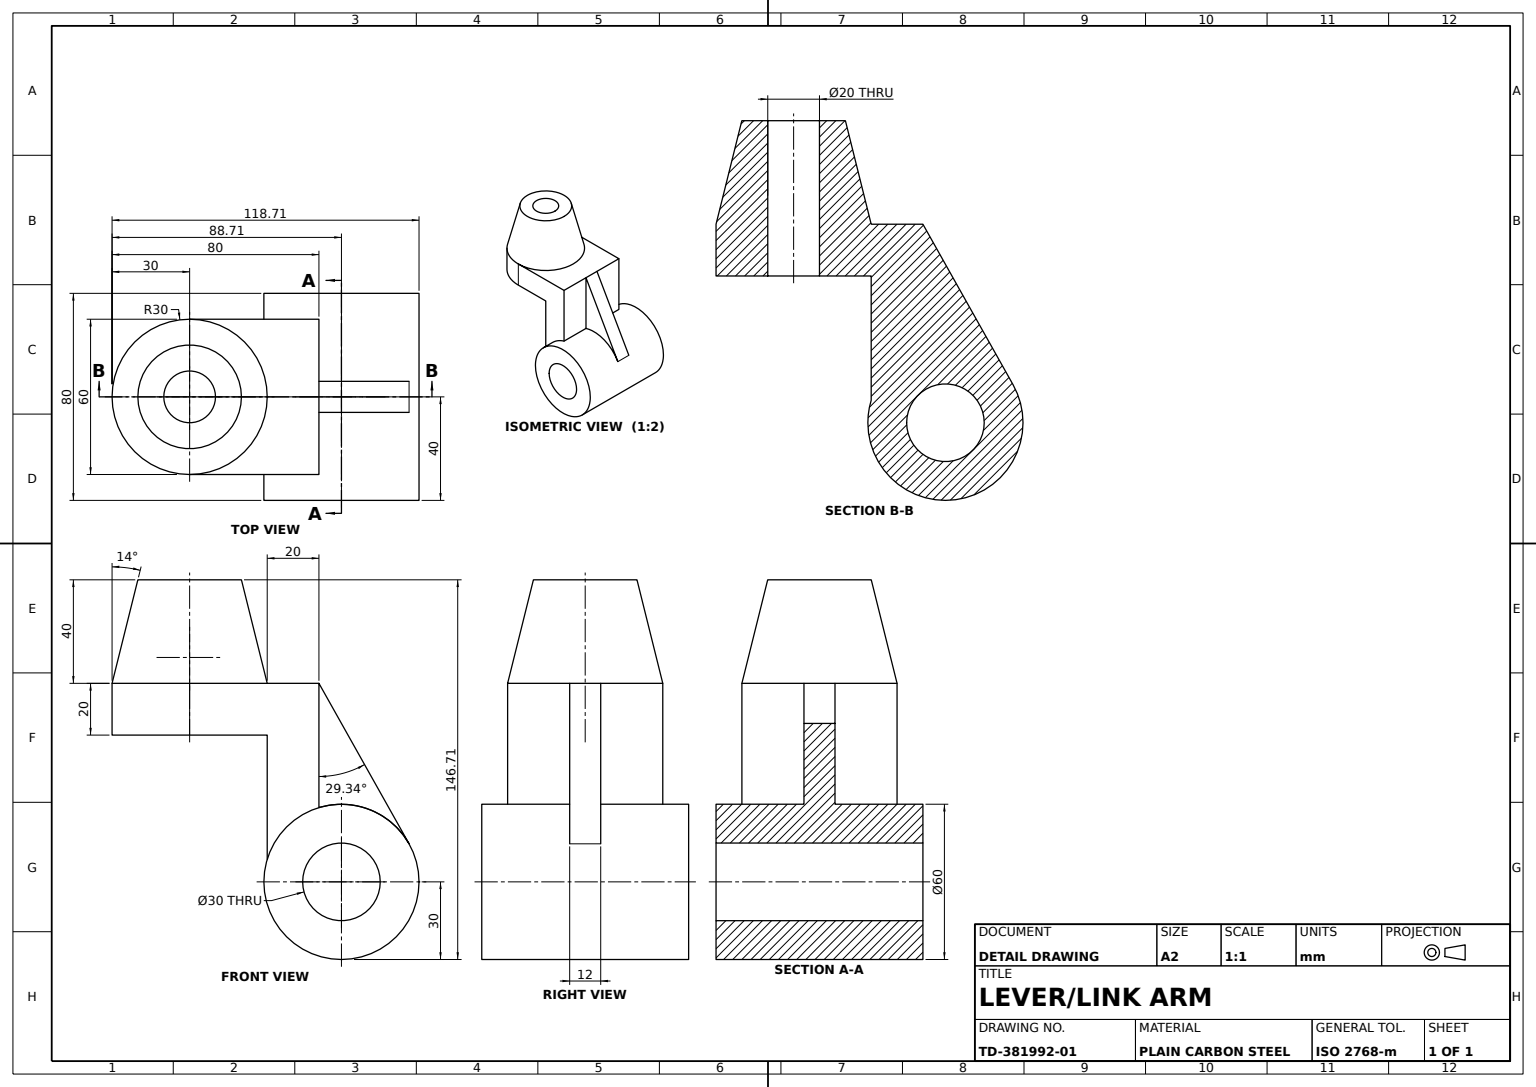
from build123d import *

# Parameters (mm, degrees)
BASE_BLOCK_SKETCH_R            = 30
BASE_BLOCK_SKETCH_R_2          = 15
BASE_BLOCK_DEPTH               = 40
ARM_DEPTH                      = 30
SUPPORT_RIB_DEPTH              = 6
PROFILE_CUT_DEPTH              = 145.415437787
DRAFTED_BOSS_SKETCH_R          = 30
DRAFTED_CYLINDRICAL_BOSS_DEPTH = 40
DRAFTED_CYLINDRICAL_BOSS_TAPER = 14
BOSS_BORE_SKETCH_R             = 10
BOSS_BORE_20_DEPTH             = 177.046816624


with BuildPart() as part:
    # Base Block Sketch → Base Block (new, symmetric)
    with BuildSketch(Plane.XY):
        Circle(BASE_BLOCK_SKETCH_R)
        Circle(BASE_BLOCK_SKETCH_R_2, mode=Mode.SUBTRACT)
    extrude(amount=BASE_BLOCK_DEPTH, both=True)

    # Arm Profile Sketch → Arm (add, symmetric)
    with BuildSketch(Plane.XY):
        with BuildLine():
            Line((-28.708286934, 8.708286934), (-28.708286934, 56.708286934))
            Line((-28.708286934, 56.708286934), (-88.708286934, 56.708286934))
            Line((-88.708286934, 56.708286934), (-88.708286934, 76.708286934))
            Line((-88.708286934, 76.708286934), (-8.708286934, 76.708286934))
            Line((-8.708286934, 76.708286934), (-8.708286934, 28.708286934))
            ThreePointArc((-8.708286934, 28.708286934), (-21.213203436, 21.213203436), (-28.708286934, 8.708286934))
        make_face()
    extrude(amount=ARM_DEPTH, both=True)

    # Support Rib Sketch → Support Rib (add, symmetric)
    with BuildSketch(Plane.XY):
        with BuildLine():
            Line((-8.708286934, 76.708286934), (26.150815657, 14.701525107))
            ThreePointArc((26.150815657, 14.701525107), (11.185159645, 27.836885668), (-8.708286934, 28.708286934))
            Line((-8.708286934, 28.708286934), (-8.708286934, 76.708286934))
        make_face()
    extrude(amount=SUPPORT_RIB_DEPTH, both=True)

    # Profile Cut Sketch → Profile Cut (cut, through all)
    with BuildSketch(Plane(origin=(0, 76.708286934, 0), x_dir=(1, 0, 0), z_dir=(0, 1, 0))):
        with BuildLine():
            Line((-88.708286934, -30), (-58.708286934, -30))
            ThreePointArc((-58.708286934, -30), (-79.921490369, -21.213203436), (-88.708286934, 0))
            Line((-88.708286934, 0), (-88.708286934, -30))
        make_face()
        with BuildLine():
            ThreePointArc((-88.708286934, 0), (-79.921490369, 21.213203436), (-58.708286934, 30))
            Line((-58.708286934, 30), (-88.708286934, 30))
            Line((-88.708286934, 30), (-88.708286934, 0))
        make_face()
    extrude(amount=-PROFILE_CUT_DEPTH, mode=Mode.SUBTRACT)

    # Drafted Boss Sketch → Drafted Cylindrical Boss (add)
    with BuildSketch(Plane(origin=(0, 76.708286934, 0), x_dir=(1, 0, 0), z_dir=(0, 1, 0))):
        with Locations((-58.708286934, 0)):
            Circle(DRAFTED_BOSS_SKETCH_R)
    extrude(amount=DRAFTED_CYLINDRICAL_BOSS_DEPTH, taper=DRAFTED_CYLINDRICAL_BOSS_TAPER)

    # Boss Bore Sketch → Boss Bore Ø20 (cut, through all)
    with BuildSketch(Plane(origin=(0, 116.708286934, 0), x_dir=(1, 0, 0), z_dir=(0, 1, 0))):
        with Locations(Location((-58.708286934, 0, 0), (0, 0, 180))):
            Circle(BOSS_BORE_SKETCH_R)
    extrude(amount=-BOSS_BORE_20_DEPTH, mode=Mode.SUBTRACT)


solid = part.part
